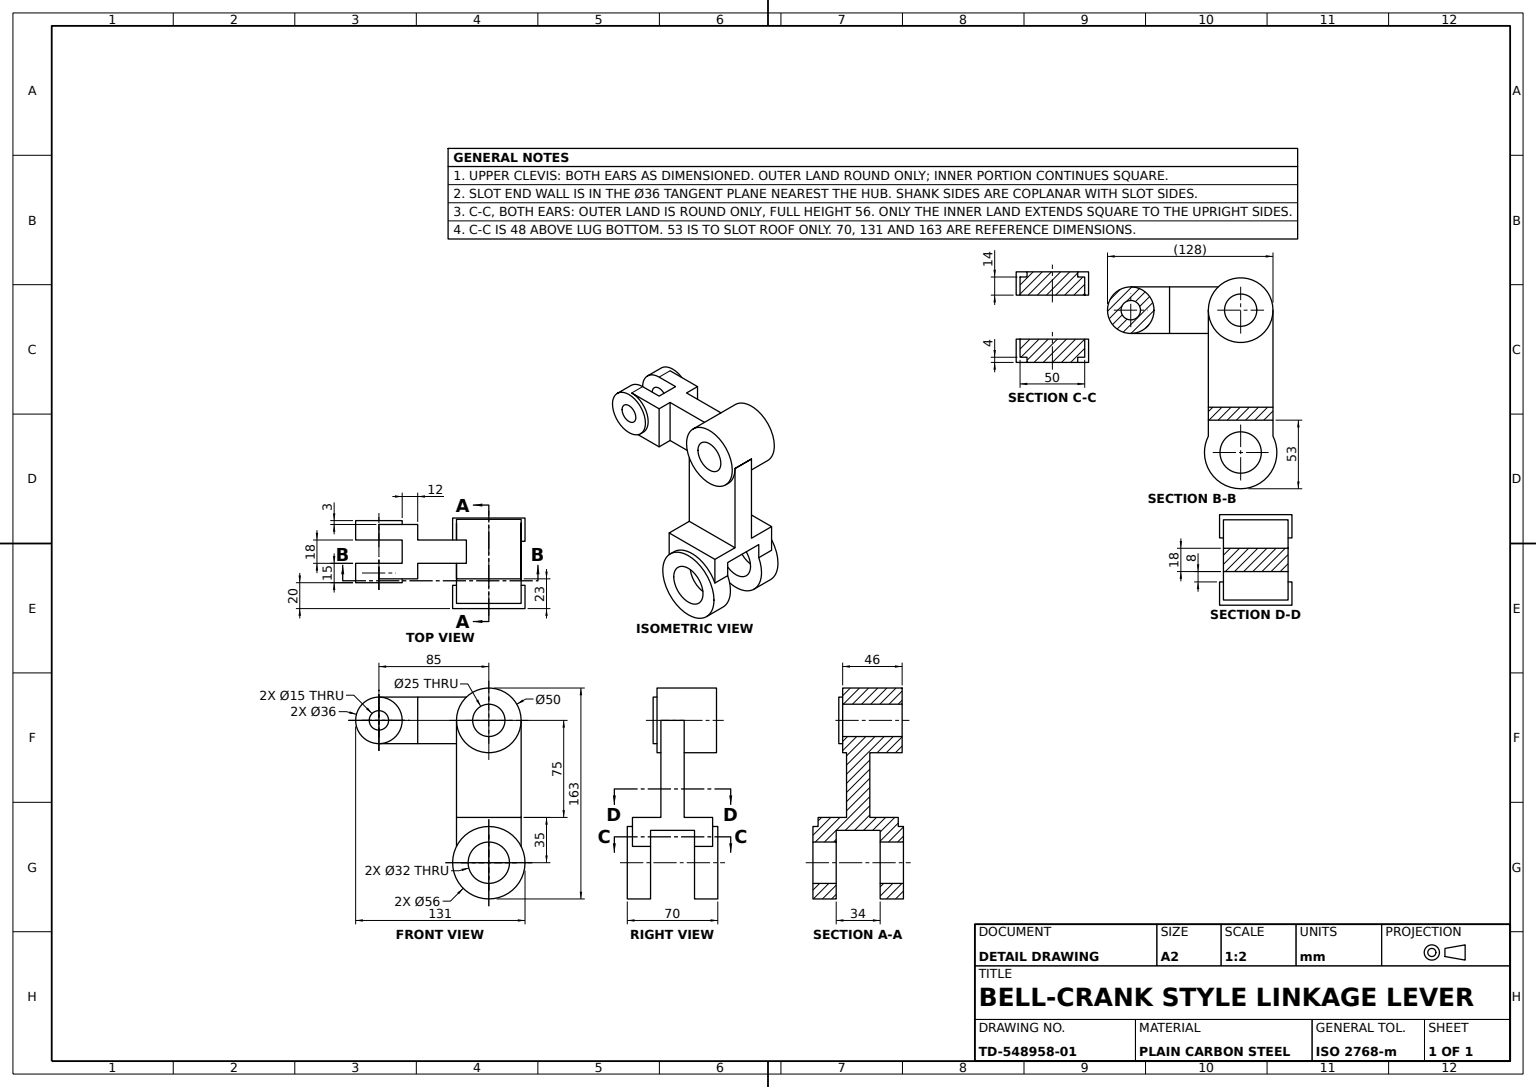
from build123d import *

# Parameters (mm, degrees)
FRONT_PIVOT_EYE_SKETCH_R        = 28
FRONT_PIVOT_EYE_SKETCH_R_2      = 16
FRONT_PIVOT_EYE_56X_32_DEPTH    = 18
REAR_PIVOT_EYE_SKETCH_R         = 28
REAR_PIVOT_EYE_SKETCH_R_2       = 16
REAR_PIVOT_EYE_56X_32_DEPTH     = 18
LOWER_CLEVIS_BLOCK_48X48_DEPTH  = 18
CLEVIS_BLOCK_RELIEF_SKETCH_W    = 3
CLEVIS_BLOCK_RELIEF_SKETCH_H    = 18
CLEVIS_BLOCK_RELIEF_CUT_DEPTH   = 80.780950107
LOWER_CLEVIS_SLOT_SKETCH_W      = 34
LOWER_CLEVIS_SLOT_SKETCH_H      = 8
LOWER_CLEVIS_SLOT_34X8_DEPTH    = 95.519839187
LOWER_WEB_PLATE_SKETCH_W        = 2.751404539
LOWER_WEB_PLATE_SKETCH_H        = 14
LOWER_WEB_PLATE_SKETCH_W_2      = 2.75570227
LOWER_WEB_PLATE_5MM_DEPTH       = 5
MAIN_ARM_SKETCH_W               = 50.004297731
MAIN_ARM_SKETCH_H               = 18
MAIN_ARM_9X18_DEPTH             = 75
UPPER_PIVOT_HUB_SKETCH_R        = 25
UPPER_PIVOT_HUB_SKETCH_R_2      = 12.5
UPPER_PIVOT_HUB_50X_25_DEPTH    = 46
HUB_BORE_SKETCH_R               = 12.5
HUB_BORE_THROUGH_CUT_25_DEPTH   = 145.723875017
UPPER_ARM_SKETCH_R              = 18
UPPER_ARM_SKETCH_R_2            = 7.5
UPPER_ARM_36X15_DEPTH           = 15
UPPER_ARM_EXTENSION_SKETCH_R    = 18
UPPER_ARM_EXTENSION_SKETCH_R_2  = 7.5
UPPER_ARM_EXTENSION_36X15_DEPTH = 15
UPPER_CLEVIS_HEAD_DEPTH         = 36
UPPER_CLEVIS_SLOT_SKETCH_R      = 12.5
UPPER_CLEVIS_SLOT_SKETCH_R_2    = 7.5
UPPER_CLEVIS_SLOT_25_DEPTH      = 177.188981887


with BuildPart() as part:
    # Front Pivot Eye Sketch → Front Pivot Eye Ø56xØ32 (new body)
    with BuildSketch(Plane.XY):
        Circle(FRONT_PIVOT_EYE_SKETCH_R)
        Circle(FRONT_PIVOT_EYE_SKETCH_R_2, mode=Mode.SUBTRACT)
    extrude(amount=-FRONT_PIVOT_EYE_56X_32_DEPTH)



with BuildPart() as body_2:
    # Rear Pivot Eye Sketch → Rear Pivot Eye Ø56xØ32 (new body)
    with BuildSketch(Plane.XY.offset(-52)):
        Circle(REAR_PIVOT_EYE_SKETCH_R)
        Circle(REAR_PIVOT_EYE_SKETCH_R_2, mode=Mode.SUBTRACT)
    extrude(amount=-REAR_PIVOT_EYE_56X_32_DEPTH)


with BuildPart() as part_1:
    add(part.part)

    add(body_2.part)  # Lower Clevis Block 48x48 merges body 2
    # Lower Clevis Block Sketch → Lower Clevis Block 48x48 (add)
    with BuildSketch(Plane(origin=(0, 35, 0), x_dir=(1, 0, 0), z_dir=(0, 1, 0))):
        Polygon((-28, 52), (-28, 66), (28, 66), (28, 18), (28, 4), (-28, 4), align=None)
    extrude(amount=-LOWER_CLEVIS_BLOCK_48X48_DEPTH)

    # Clevis Block Relief Sketch → Clevis Block Relief Cut (cut, through all)
    with BuildSketch(Plane.XY.offset(-4)):
        with Locations((-26.5, 26)):
            Rectangle(CLEVIS_BLOCK_RELIEF_SKETCH_W, CLEVIS_BLOCK_RELIEF_SKETCH_H)
        Polygon((28, 17), (25.124297731, 17), (25.004297731, 17), (25.004297731, 35), (28, 35), align=None)
    extrude(amount=-CLEVIS_BLOCK_RELIEF_CUT_DEPTH, mode=Mode.SUBTRACT)

    # Lower Clevis Slot Sketch → Lower Clevis Slot 34x8 (cut, through all)
    with BuildSketch(Plane.ZY.offset(25)):
        with Locations((-35, 21)):
            Rectangle(LOWER_CLEVIS_SLOT_SKETCH_W, LOWER_CLEVIS_SLOT_SKETCH_H)
    extrude(amount=-LOWER_CLEVIS_SLOT_34X8_DEPTH, mode=Mode.SUBTRACT)

    # Lower Web Plate Sketch → Lower Web Plate 5mm (add)
    with BuildSketch(Plane.XZ.offset(-17)):
        with Locations((-23.624297731, -59)):
            Rectangle(LOWER_WEB_PLATE_SKETCH_W, LOWER_WEB_PLATE_SKETCH_H)
        with Locations((-23.624297731, -11)):
            Rectangle(LOWER_WEB_PLATE_SKETCH_W, LOWER_WEB_PLATE_SKETCH_H)
        with Locations((23.626446596, -11)):
            Rectangle(LOWER_WEB_PLATE_SKETCH_W_2, LOWER_WEB_PLATE_SKETCH_H)
        with Locations((23.626446596, -59)):
            Rectangle(LOWER_WEB_PLATE_SKETCH_W_2, LOWER_WEB_PLATE_SKETCH_H)
    extrude(amount=LOWER_WEB_PLATE_5MM_DEPTH)

    # Main Arm Sketch → Main Arm 9x18 (add)
    with BuildSketch(Plane(origin=(0, 35, 0), x_dir=(1, 0, 0), z_dir=(0, 1, 0))):
        with Locations((0.002148866, 35)):
            Rectangle(MAIN_ARM_SKETCH_W, MAIN_ARM_SKETCH_H)
    extrude(amount=MAIN_ARM_9X18_DEPTH)

    # Upper Pivot Hub Sketch → Upper Pivot Hub Ø50xØ25 (add)
    with BuildSketch(Plane.XY.offset(-23)):
        with Locations((0.002148865, 110)):
            Circle(UPPER_PIVOT_HUB_SKETCH_R)
        with Locations((0.002148865, 110)):
            Circle(UPPER_PIVOT_HUB_SKETCH_R_2, mode=Mode.SUBTRACT)
    extrude(amount=-UPPER_PIVOT_HUB_50X_25_DEPTH)

    # Hub Bore Sketch → Hub Bore Through Cut Ø25 (cut, through all)
    with BuildSketch(Plane.XY.offset(-26)):
        with Locations((0.002148865, 110)):
            Circle(HUB_BORE_SKETCH_R)
    extrude(amount=-HUB_BORE_THROUGH_CUT_25_DEPTH, mode=Mode.SUBTRACT)



with BuildPart() as body_2_2:
    # Upper Arm Sketch → Upper Arm 36x15 (new body)
    with BuildSketch(Plane.XY.offset(-20)):
        with Locations((-84.997851135, 110)):
            Circle(UPPER_ARM_SKETCH_R)
        with Locations((-84.997851135, 110)):
            Circle(UPPER_ARM_SKETCH_R_2, mode=Mode.SUBTRACT)
    extrude(amount=-UPPER_ARM_36X15_DEPTH)


with BuildPart() as body_3:
    # Upper Arm Extension Sketch → Upper Arm Extension 36x15 (new body)
    with BuildSketch(Plane.XY.offset(-53)):
        with Locations((-84.997851135, 110)):
            Circle(UPPER_ARM_EXTENSION_SKETCH_R)
        with Locations((-84.997851135, 110)):
            Circle(UPPER_ARM_EXTENSION_SKETCH_R_2, mode=Mode.SUBTRACT)
    extrude(amount=-UPPER_ARM_EXTENSION_36X15_DEPTH)


with BuildPart() as part_2:
    add(part_1.part)

    add(body_2_2.part)  # Upper Clevis Head merges body 2 2

    add(body_3.part)  # Upper Clevis Head merges body 3
    # Upper Clevis Head Sketch → Upper Clevis Head (add)
    with BuildSketch(Plane(origin=(0, 128, 0), x_dir=(1, 0, 0), z_dir=(0, 1, 0))):
        Polygon((-84.997851135, 53), (-84.997851135, 65), (-54.997851135, 65), (-54.997851135, 53), (-4.745708578, 53), (-4.745708578, 35), (-54.997851135, 35), (-54.997851135, 23), (-84.997851135, 23), (-84.997851135, 35), (-66.997851135, 35), (-66.997851135, 53), align=None)
    extrude(amount=-UPPER_CLEVIS_HEAD_DEPTH)

    # Upper Clevis Slot Sketch → Upper Clevis Slot 25 (cut, through all)
    with BuildSketch(Plane.XY.offset(-23)):
        with Locations((0.002148865, 110)):
            Circle(UPPER_CLEVIS_SLOT_SKETCH_R)
        with Locations((-84.997851135, 110)):
            Circle(UPPER_CLEVIS_SLOT_SKETCH_R_2)
    extrude(amount=-UPPER_CLEVIS_SLOT_25_DEPTH, mode=Mode.SUBTRACT)


solid = part_2.part
